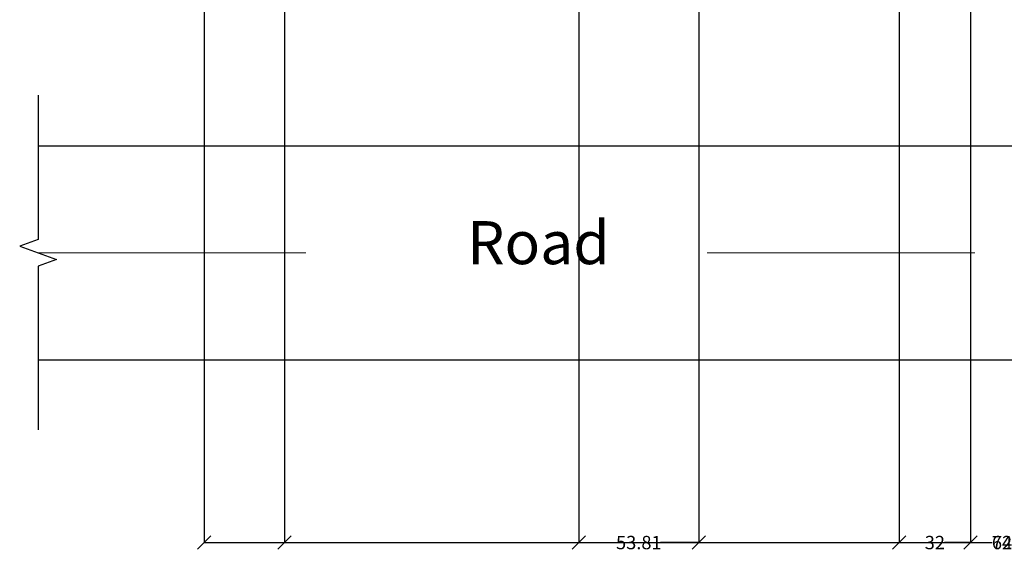
# Model space of a CAD drawing. Units: inches. Extents: x -1198 to -69, y -512 to 437.
# Tile 1 of 50: x -1137 to -696, y -512 to -273. Entities that reach past the tile are written whole.
import ezdxf

# ---------------------------------------------------------------- set-up
doc = ezdxf.new("R2010")
doc.units = ezdxf.units.IN
doc.header["$MEASUREMENT"] = 0
doc.linetypes.add('ACAD_ISO03W100', pattern=[30, 12, -18])
for name, color, linetype, lineweight in [('A-ANNO-DIMS', 2, 'Continuous', 18), ('A-ANNO-TEXT', 7, 'Continuous', 25), ('C-ROAD', 7, 'Continuous', 25), ('C-ROAD-CNTR', 7, 'ACAD_ISO03W100', 18)]:
    doc.layers.add(name, color=color, linetype=linetype, lineweight=lineweight)
doc.styles.get("Standard").update_dxf_attribs({"font": 'arial.ttf'})
doc.dimstyles.get("Standard").update_dxf_attribs({"dimtxt": 6, "dimasz": 6, "dimexe": 0.18, "dimexo": 0.0625, "dimgap": 0.09, "dimtad": 0, "dimtih": 1, "dimtoh": 1, "dimdec": 0, "dimzin": 0, "dimdsep": 46, "dimlunit": 4, "dimtxsty": 'Standard', "dimblk": 'OBLIQUE', "dimcen": 0.09, "dimadec": 0, "dimazin": 0, "dimtfac": 1, "dimtdec": 0, "dimtofl": 0, "dimtmove": 0, "dimatfit": 3, "dimfxl": 1, "dimtolj": 1, "dimtzin": 0, "dimarcsym": 0})

# ---------------------------------------------------------------- blocks, each defined once
blk = doc.blocks.new('_Oblique')
at = {"color": 0, "linetype": 'ByBlock', "lineweight": -2}
blk.add_line((-0.5, -0.5), (0.5, 0.5), dxfattribs=at)
blk = doc.blocks.new('*D60')
at = {"layer": 'A-ANNO-DIMS', "color": 0, "lineweight": -2, "ltscale": 10, "transparency": 16777216}
for p, q in [((-1054.75, -264.83), (-1054.75, -507.84)), ((-334.75, -264.83), (-334.75, -507.84)), ((-1054.75, -507.66), (-701.43, -507.66)), ((-334.75, -507.66), (-688.07, -507.66))]:
    blk.add_line(p, q, dxfattribs=at)
at = {"layer": 'DEFPOINTS', "color": 0, "ltscale": 10, "transparency": 16777216}
for p in [(-1054.75, -264.77), (-334.75, -264.77), (-334.75, -507.66)]:
    blk.add_point(p, dxfattribs=at)
at = {"layer": 'A-ANNO-DIMS', "color": 0, "lineweight": -2, "ltscale": 10, "transparency": 16777216, "xscale": 6, "yscale": 6, "zscale": 6, "rotation": 180}
blk.add_blockref('_Oblique', (-1054.75, -507.66), dxfattribs=at)
at = {"layer": 'A-ANNO-DIMS', "color": 0, "lineweight": -2, "ltscale": 10, "transparency": 16777216, "xscale": 6, "yscale": 6, "zscale": 6}
blk.add_blockref('_Oblique', (-334.75, -507.66), dxfattribs=at)
at = {"layer": 'A-ANNO-DIMS', "color": 0, "ltscale": 10, "transparency": 16777216, "insert": (-694.75, -507.66), "char_height": 6, "attachment_point": 5}
blk.add_mtext('\\A1;720', dxfattribs=at)
blk = doc.blocks.new('*D62')
at = {"layer": 'A-ANNO-DIMS', "color": 0, "lineweight": -2, "ltscale": 10, "transparency": 16777216}
for p, q in [((-1018.75, -228.83), (-1018.75, -507.84)), ((-370.75, -228.83), (-370.75, -507.84)), ((-1018.75, -507.66), (-701.49, -507.66)), ((-370.75, -507.66), (-688.01, -507.66))]:
    blk.add_line(p, q, dxfattribs=at)
at = {"layer": 'DEFPOINTS', "color": 0, "ltscale": 10, "transparency": 16777216}
for p in [(-1018.75, -228.77), (-370.75, -228.77), (-370.75, -507.66)]:
    blk.add_point(p, dxfattribs=at)
at = {"layer": 'A-ANNO-DIMS', "color": 0, "lineweight": -2, "ltscale": 10, "transparency": 16777216, "xscale": 6, "yscale": 6, "zscale": 6, "rotation": 180}
blk.add_blockref('_Oblique', (-1018.75, -507.66), dxfattribs=at)
at = {"layer": 'A-ANNO-DIMS', "color": 0, "lineweight": -2, "ltscale": 10, "transparency": 16777216, "xscale": 6, "yscale": 6, "zscale": 6}
blk.add_blockref('_Oblique', (-370.75, -507.66), dxfattribs=at)
at = {"layer": 'A-ANNO-DIMS', "color": 0, "ltscale": 10, "transparency": 16777216, "insert": (-694.75, -507.66), "char_height": 6, "attachment_point": 5}
blk.add_mtext('\\A1;648', dxfattribs=at)
blk = doc.blocks.new('*D72')
at = {"layer": 'A-ANNO-DIMS', "color": 0, "lineweight": -2, "ltscale": 10, "transparency": 16777216}
for p, q in [((-743.13, -44.33), (-743.13, -507.84)), ((-711.13, -44.33), (-711.13, -507.84)), ((-743.13, -507.66), (-731.49, -507.66)), ((-711.13, -507.66), (-722.78, -507.66))]:
    blk.add_line(p, q, dxfattribs=at)
at = {"layer": 'DEFPOINTS', "color": 0, "ltscale": 10, "transparency": 16777216}
for p in [(-743.13, -44.27), (-711.13, -44.27), (-711.13, -507.66)]:
    blk.add_point(p, dxfattribs=at)
at = {"layer": 'A-ANNO-DIMS', "color": 0, "lineweight": -2, "ltscale": 10, "transparency": 16777216, "xscale": 6, "yscale": 6, "zscale": 6, "rotation": 180}
blk.add_blockref('_Oblique', (-743.13, -507.66), dxfattribs=at)
at = {"layer": 'A-ANNO-DIMS', "color": 0, "lineweight": -2, "ltscale": 10, "transparency": 16777216, "xscale": 6, "yscale": 6, "zscale": 6}
blk.add_blockref('_Oblique', (-711.13, -507.66), dxfattribs=at)
at = {"layer": 'A-ANNO-DIMS', "color": 0, "ltscale": 10, "transparency": 16777216, "insert": (-727.13, -507.66), "char_height": 6, "attachment_point": 5}
blk.add_mtext('\\A1;32', dxfattribs=at)
blk = doc.blocks.new('*D77')
at = {"layer": 'A-ANNO-DIMS', "color": 0, "lineweight": -2, "ltscale": 10, "transparency": 16777216}
for p, q in [((-886.75, -44.33), (-886.75, -507.84)), ((-832.94, -44.33), (-832.94, -507.84)), ((-886.75, -507.66), (-869.48, -507.66)), ((-832.94, -507.66), (-850.21, -507.66))]:
    blk.add_line(p, q, dxfattribs=at)
at = {"layer": 'DEFPOINTS', "color": 0, "ltscale": 10, "transparency": 16777216}
for p in [(-886.75, -44.27), (-832.94, -44.27), (-832.94, -507.66)]:
    blk.add_point(p, dxfattribs=at)
at = {"layer": 'A-ANNO-DIMS', "color": 0, "lineweight": -2, "ltscale": 10, "transparency": 16777216, "xscale": 6, "yscale": 6, "zscale": 6, "rotation": 180}
blk.add_blockref('_Oblique', (-886.75, -507.66), dxfattribs=at)
at = {"layer": 'A-ANNO-DIMS', "color": 0, "lineweight": -2, "ltscale": 10, "transparency": 16777216, "xscale": 6, "yscale": 6, "zscale": 6}
blk.add_blockref('_Oblique', (-832.94, -507.66), dxfattribs=at)
at = {"layer": 'A-ANNO-DIMS', "color": 0, "ltscale": 10, "transparency": 16777216, "insert": (-859.85, -507.66), "char_height": 6, "attachment_point": 5}
blk.add_mtext('\\A1;53.81', dxfattribs=at)

msp = doc.modelspace()

# ---------------------------------------------------------------- linework, layer by layer
at = {"layer": 'C-ROAD', "ltscale": 10}
for p, q in [((-1129.1823, -329.6039), (-264.1167, -329.6039)), ((-1129.1823, -425.6039), (-168.1167, -425.6039))]:
    msp.add_line(p, q, dxfattribs=at)
msp.add_lwpolyline([(-1129.1823, -306.8434), (-1129.1823, -371.6039), (-1137.4248, -374.6039), (-1120.9399, -380.6039), (-1129.1823, -383.6039), (-1129.1823, -457.0552)], dxfattribs=at)
at = {"layer": 'C-ROAD-CNTR', "ltscale": 10}
msp.add_line((-1129.1823, -377.6039), (-168.1167, -377.6039), dxfattribs=at)

# ---------------------------------------------------------------- texts
at = {"layer": 'A-ANNO-TEXT', "ltscale": 10, "insert": (-936.7913, -363.3693), "char_height": 19.32196, "attachment_point": 1}
msp.add_mtext_dynamic_manual_height_columns('Road', width=186.703358, gutter_width=96.6098, heights=[0], dxfattribs=at)

# ---------------------------------------------------------------- dimensions: what is measured, and where the dimension line sits
at = {"layer": 'A-ANNO-DIMS', "ltscale": 10}
for base, p1, p2, override, picture, middle in [((-832.9414, -507.6552), (-886.7509, -44.2723), (-832.9414, -44.2723), {"dimdec": 2, "dimlfac": 1, "dimrnd": 0, "dimzin": 0, "dimdsep": 46, "dimlunit": 2}, '*D77', (-859.8461, -507.6552)), ((-711.1319, -507.6552), (-743.1319, -44.2723), (-711.1319, -44.2723), {"dimdec": 0, "dimlfac": 1, "dimrnd": 0, "dimzin": 0, "dimdsep": 46, "dimlunit": 2}, '*D72', (-727.1319, -507.6552)), ((-370.7509, -507.6552), (-1018.7509, -228.7723), (-370.7509, -228.7723), {"dimdec": 0, "dimlfac": 1, "dimrnd": 0, "dimzin": 0, "dimdsep": 46, "dimlunit": 2}, '*D62', (-694.7509, -507.6552)), ((-334.7509, -507.6552), (-1054.7509, -264.7723), (-334.7509, -264.7723), {"dimdec": 0, "dimlfac": 1, "dimrnd": 0, "dimzin": 0, "dimdsep": 46, "dimlunit": 2}, '*D60', (-694.7509, -507.6552))]:
    dim = msp.add_linear_dim(base=base, p1=p1, p2=p2, dimstyle='Standard', override=override, dxfattribs=at)
    dim.commit()
    dim.dimension.update_dxf_attribs({"geometry": picture, "text_midpoint": middle})

doc.saveas('drawing.dxf')
